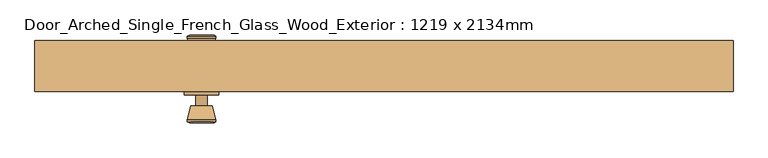
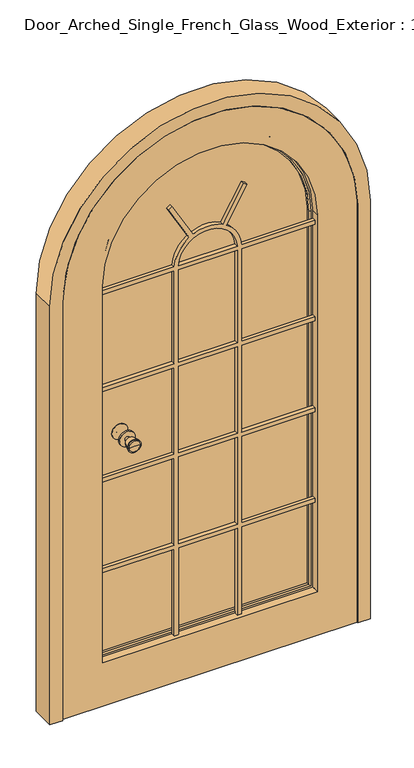
"""IFC4 building model written with IfcOpenShell, lengths in millimetres: door geometry, Door_Arched_Single_French_Glass_Wood_Exterior : 1219 x 2134mm."""

from ifc_helpers import new_model, si_unit, point, frame, frame_2d, origin, place, context, project, spatial, polyline, circle_curve, ellipse_curve, trimmed, segment, composite_curve, outline, extrude, source, transform, mapped, element, save
from ifc_brep_helpers import plane_surface, cylinder_surface, revolved_surface, advanced_brep


def door_arched_single_french_glass_wood_exterior_1219_x_2134mm_7a906126(model_context):
    return source(origin(), model_context, "Body", "SolidModel", [
        advanced_brep(
        [(-318.5, -5.7, 1050.0), (-308.5, -5.7, 1050.0), (-328.5, -5.7, 1050.0), (-298.0241324, -54.7, 1050.0), (-318.5, -54.7, 1050.0), (-338.9758676, -54.7, 1050.0), (-293.5, -52.8721319, 1050.0), (-343.5, -52.8721319, 1050.0), (-293.5, -49.4084537, 1050.0), (-343.5, -49.4084537, 1050.0), (-299.863764, -24.7, 1050.0), (-337.136236, -24.7, 1050.0), (-308.5, -24.7, 1050.0), (-328.5, -24.7, 1050.0)],
        [
            (0, 1),
            (1, 2, circle_curve(frame((-318.5, -5.7, 1050.0), z_axis=(0.0, 1.0, 0.0), x_axis=(-1.0, 0.0, 0.0)), 10.0)),
            (2, 0),
            (2, 1, circle_curve(frame((-318.5, -5.7, 1050.0), z_axis=(0.0, 1.0, 0.0), x_axis=(-1.0, 0.0, 0.0)), 10.0)),
            (3, 4),
            (4, 5),
            (5, 3, circle_curve(frame((-318.5, -54.7, 1050.0), z_axis=(0.0, -1.0, 0.0), x_axis=(-1.0, 0.0, 0.0)), 20.4758676)),
            (3, 5, circle_curve(frame((-318.5, -54.7, 1050.0), z_axis=(0.0, -1.0, 0.0), x_axis=(-1.0, 0.0, 0.0)), 20.4758676)),
            (6, 3),
            (5, 7),
            (7, 6, circle_curve(frame((-318.5, -52.8721319, 1050.0), z_axis=(0.0, -1.0, 0.0), x_axis=(-1.0, 0.0, 0.0)), 25.0)),
            (6, 7, circle_curve(frame((-318.5, -52.8721319, 1050.0), z_axis=(0.0, -1.0, 0.0), x_axis=(-1.0, 0.0, 0.0)), 25.0)),
            (8, 6),
            (7, 9),
            (9, 8, circle_curve(frame((-318.5, -49.4084537, 1050.0), z_axis=(0.0, -1.0, 0.0), x_axis=(-1.0, 0.0, 0.0)), 25.0)),
            (8, 9, circle_curve(frame((-318.5, -49.4084537, 1050.0), z_axis=(0.0, -1.0, 0.0), x_axis=(-1.0, 0.0, 0.0)), 25.0)),
            (10, 8),
            (9, 11),
            (11, 10, circle_curve(frame((-318.5, -24.7, 1050.0), z_axis=(0.0, -1.0, 0.0), x_axis=(-1.0, 0.0, 0.0)), 18.636236)),
            (10, 11, circle_curve(frame((-318.5, -24.7, 1050.0), z_axis=(0.0, -1.0, 0.0), x_axis=(-1.0, 0.0, 0.0)), 18.636236)),
            (12, 10),
            (11, 13),
            (13, 12, circle_curve(frame((-318.5, -24.7, 1050.0), z_axis=(0.0, -1.0, 0.0), x_axis=(-1.0, 0.0, 0.0)), 10.0)),
            (12, 13, circle_curve(frame((-318.5, -24.7, 1050.0), z_axis=(0.0, -1.0, 0.0), x_axis=(-1.0, 0.0, 0.0)), 10.0)),
            (1, 12),
            (13, 2),
        ],
        [
            plane_surface(frame((-318.5, -5.7, 1050.0), z_axis=(0.0, 1.0, 0.0), x_axis=(-1.0, 0.0, 0.0))),
            plane_surface(frame((-318.5, -54.7, 1050.0), z_axis=(0.0, -1.0, 0.0), x_axis=(-1.0, 0.0, 0.0))),
            revolved_surface(polyline([(-338.9758676, -54.7, 1050.0), (-343.5, -52.8721319, 1050.0)]), (-318.5, -5.7, 1050.0), (0.0, 1.0, 0.0)),
            cylinder_surface(frame((-318.5, -5.7, 1050.0), z_axis=(0.0, 1.0, 0.0), x_axis=(-1.0, 0.0, 0.0)), 25.0),
            revolved_surface(polyline([(-343.5, -49.4084537, 1050.0), (-337.136236, -24.7, 1050.0)]), (-318.5, -5.7, 1050.0), (0.0, 1.0, 0.0)),
            plane_surface(frame((-318.5, -24.7, 1050.0), z_axis=(0.0, 1.0, 0.0), x_axis=(-1.0, 0.0, 0.0))),
            cylinder_surface(frame((-318.5, -5.7, 1050.0), z_axis=(0.0, 1.0, 0.0), x_axis=(-1.0, 0.0, 0.0)), 10.0),
        ],
        [
            (0, [[1, 2, 3]]),
            (0, [[-3, 4, -1]]),
            (1, [[5, 6, 7]]),
            (1, [[-6, -5, 8]]),
            (2, [[9, -7, 10, 11]]),
            (2, [[-10, -8, -9, 12]]),
            (3, [[13, -11, 14, 15]]),
            (3, [[-14, -12, -13, 16]]),
            (4, [[17, -15, 18, 19]]),
            (4, [[-18, -16, -17, 20]]),
            (5, [[21, -19, 22, 23]]),
            (5, [[-22, -20, -21, 24]]),
            (6, [[25, -23, 26, -2]]),
            (6, [[-26, -24, -25, -4]]),
        ],
    ),
        extrude(outline(composite_curve([segment(trimmed(circle_curve(frame_2d((1050.0, -318.5)), 30.0), [point((1050.0, -348.5))], [point((1050.0, -288.5))], False, "CARTESIAN"), True, "CONTINUOUS"), segment(trimmed(circle_curve(frame_2d((1050.0, -318.5)), 30.0), [point((1050.0, -288.5))], [point((1050.0, -348.5))], False, "CARTESIAN"), True, "CONTINUOUS")], self_intersect=False)), frame((0.0, -5.7, 0.0), z_axis=(0.0, 1.0, 0.0), x_axis=(0.0, 0.0, 1.0)), (0.0, 0.0, 1.0), 6.0),
        advanced_brep(
        [(-318.5, 50.3, 1050.0), (-328.5, 50.3, 1050.0), (-308.5, 50.3, 1050.0), (-298.0241324, 99.3, 1050.0), (-338.9758676, 99.3, 1050.0), (-318.5, 99.3, 1050.0), (-293.5, 97.4721319, 1050.0), (-343.5, 97.4721319, 1050.0), (-293.5, 94.0084537, 1050.0), (-343.5, 94.0084537, 1050.0), (-299.863764, 69.3, 1050.0), (-337.136236, 69.3, 1050.0), (-308.5, 69.3, 1050.0), (-328.5, 69.3, 1050.0)],
        [
            (0, 1),
            (1, 2, circle_curve(frame((-318.5, 50.3, 1050.0), z_axis=(0.0, -1.0, 0.0), x_axis=(-1.0, 0.0, 0.0)), 10.0)),
            (2, 0),
            (2, 1, circle_curve(frame((-318.5, 50.3, 1050.0), z_axis=(0.0, -1.0, 0.0), x_axis=(-1.0, 0.0, 0.0)), 10.0)),
            (3, 4, circle_curve(frame((-318.5, 99.3, 1050.0), z_axis=(0.0, 1.0, 0.0), x_axis=(-1.0, 0.0, 0.0)), 20.4758676)),
            (4, 5),
            (5, 3),
            (4, 3, circle_curve(frame((-318.5, 99.3, 1050.0), z_axis=(0.0, 1.0, 0.0), x_axis=(-1.0, 0.0, 0.0)), 20.4758676)),
            (6, 7, circle_curve(frame((-318.5, 97.4721319, 1050.0), z_axis=(0.0, 1.0, 0.0), x_axis=(-1.0, 0.0, 0.0)), 25.0)),
            (7, 4),
            (3, 6),
            (7, 6, circle_curve(frame((-318.5, 97.4721319, 1050.0), z_axis=(0.0, 1.0, 0.0), x_axis=(-1.0, 0.0, 0.0)), 25.0)),
            (8, 9, circle_curve(frame((-318.5, 94.0084537, 1050.0), z_axis=(0.0, 1.0, 0.0), x_axis=(-1.0, 0.0, 0.0)), 25.0)),
            (9, 7),
            (6, 8),
            (9, 8, circle_curve(frame((-318.5, 94.0084537, 1050.0), z_axis=(0.0, 1.0, 0.0), x_axis=(-1.0, 0.0, 0.0)), 25.0)),
            (10, 11, circle_curve(frame((-318.5, 69.3, 1050.0), z_axis=(0.0, 1.0, 0.0), x_axis=(-1.0, 0.0, 0.0)), 18.636236)),
            (11, 9),
            (8, 10),
            (11, 10, circle_curve(frame((-318.5, 69.3, 1050.0), z_axis=(0.0, 1.0, 0.0), x_axis=(-1.0, 0.0, 0.0)), 18.636236)),
            (12, 13, circle_curve(frame((-318.5, 69.3, 1050.0), z_axis=(0.0, 1.0, 0.0), x_axis=(-1.0, 0.0, 0.0)), 10.0)),
            (13, 11),
            (10, 12),
            (13, 12, circle_curve(frame((-318.5, 69.3, 1050.0), z_axis=(0.0, 1.0, 0.0), x_axis=(-1.0, 0.0, 0.0)), 10.0)),
            (1, 13),
            (12, 2),
        ],
        [
            plane_surface(frame((-318.5, 50.3, 1050.0), z_axis=(0.0, -1.0, 0.0), x_axis=(-1.0, 0.0, 0.0))),
            plane_surface(frame((-318.5, 99.3, 1050.0), z_axis=(0.0, 1.0, 0.0), x_axis=(-1.0, 0.0, 0.0))),
            revolved_surface(polyline([(-338.9758676, 99.3, 1050.0), (-343.5, 97.4721319, 1050.0)]), (-318.5, 50.3, 1050.0), (0.0, -1.0, 0.0)),
            cylinder_surface(frame((-318.5, 50.3, 1050.0), z_axis=(0.0, -1.0, 0.0), x_axis=(-1.0, 0.0, 0.0)), 25.0),
            revolved_surface(polyline([(-343.5, 94.0084537, 1050.0), (-337.136236, 69.3, 1050.0)]), (-318.5, 50.3, 1050.0), (0.0, -1.0, 0.0)),
            plane_surface(frame((-318.5, 69.3, 1050.0), z_axis=(0.0, -1.0, 0.0), x_axis=(-1.0, 0.0, 0.0))),
            cylinder_surface(frame((-318.5, 50.3, 1050.0), z_axis=(0.0, -1.0, 0.0), x_axis=(-1.0, 0.0, 0.0)), 10.0),
        ],
        [
            (0, [[1, 2, 3]]),
            (0, [[-3, 4, -1]]),
            (1, [[5, 6, 7]]),
            (1, [[8, -7, -6]]),
            (2, [[9, 10, -5, 11]]),
            (2, [[12, -11, -8, -10]]),
            (3, [[13, 14, -9, 15]]),
            (3, [[16, -15, -12, -14]]),
            (4, [[17, 18, -13, 19]]),
            (4, [[20, -19, -16, -18]]),
            (5, [[21, 22, -17, 23]]),
            (5, [[24, -23, -20, -22]]),
            (6, [[-2, 25, -21, 26]]),
            (6, [[-4, -26, -24, -25]]),
        ],
    ),
        extrude(outline(composite_curve([segment(trimmed(circle_curve(frame_2d((1050.0, -318.5)), 30.0), [point((1050.0, -348.5))], [point((1050.0, -288.5))], False, "CARTESIAN"), True, "CONTINUOUS"), segment(trimmed(circle_curve(frame_2d((1050.0, -318.5)), 30.0), [point((1050.0, -288.5))], [point((1050.0, -348.5))], False, "CARTESIAN"), True, "CONTINUOUS")], self_intersect=False)), frame((0.0, 44.3, 0.0), z_axis=(0.0, 1.0, 0.0), x_axis=(0.0, 0.0, 1.0)), (0.0, 0.0, 1.0), 6.0),
        advanced_brep(
        [(539.1, 89.3, 0.0), (609.6, 89.3, 0.0), (609.6, 0.3, 0.0), (561.1, 0.3, 0.0), (561.1, 47.3, 0.0), (539.1, 47.3, 0.0), (539.1, 89.3, 1678.6), (-539.1, 89.3, 1678.6), (-539.1, 89.3, 0.0), (-609.6, 89.3, 0.0), (-609.6, 89.3, 1678.6), (609.6, 89.3, 1678.6), (609.6, 0.3, 1678.6), (-609.6, 0.3, 1678.6), (-609.6, 0.3, 0.0), (-561.1, 0.3, 0.0), (-561.1, 0.3, 1678.6), (561.1, 0.3, 1678.6), (561.1, 47.3, 1678.6), (-561.1, 47.3, 1678.6), (-561.1, 47.3, 0.0), (-539.1, 47.3, 0.0), (-539.1, 47.3, 1678.6), (539.1, 47.3, 1678.6)],
        [
            (0, 1),
            (1, 2),
            (2, 3),
            (3, 4),
            (4, 5),
            (5, 0),
            (0, 6),
            (6, 7, circle_curve(frame((0.0, 89.3, 1678.6), z_axis=(0.0, -1.0, 0.0), x_axis=(1.0, 0.0, 0.0)), 539.1)),
            (7, 8),
            (8, 9),
            (9, 10),
            (10, 11, circle_curve(frame((0.0, 89.3, 1678.6), z_axis=(0.0, 1.0, 0.0), x_axis=(1.0, 0.0, 0.0)), 609.6)),
            (11, 1),
            (11, 12),
            (12, 2),
            (12, 13, circle_curve(frame((0.0, 0.3, 1678.6), z_axis=(0.0, -1.0, 0.0), x_axis=(1.0, 0.0, 0.0)), 609.6)),
            (13, 14),
            (14, 15),
            (15, 16),
            (16, 17, circle_curve(frame((0.0, 0.3, 1678.6), z_axis=(0.0, 1.0, 0.0), x_axis=(1.0, 0.0, 0.0)), 561.1)),
            (17, 3),
            (17, 18),
            (18, 4),
            (18, 19, circle_curve(frame((0.0, 47.3, 1678.6), z_axis=(0.0, -1.0, 0.0), x_axis=(1.0, 0.0, 0.0)), 561.1)),
            (19, 20),
            (20, 21),
            (21, 22),
            (22, 23, circle_curve(frame((0.0, 47.3, 1678.6), z_axis=(0.0, 1.0, 0.0), x_axis=(1.0, 0.0, 0.0)), 539.1)),
            (23, 5),
            (23, 6),
            (7, 22),
            (21, 8),
            (20, 15),
            (14, 9),
            (13, 10),
            (19, 16),
        ],
        [
            plane_surface(frame((603.1, -9.1123976, 0.0), z_axis=(0.0, 0.0, -1.0), x_axis=(1.0, 0.0, 0.0))),
            plane_surface(frame((539.1, 89.3, 0.0), z_axis=(0.0, 1.0, 0.0), x_axis=(0.0, 0.0, 1.0))),
            plane_surface(frame((609.6, 89.3, 0.0), z_axis=(1.0, 0.0, 0.0), x_axis=(0.0, 0.0, 1.0))),
            plane_surface(frame((609.6, 0.3, 0.0), z_axis=(0.0, -1.0, 0.0), x_axis=(0.0, 0.0, 1.0))),
            plane_surface(frame((561.1, 0.3, 0.0), z_axis=(-1.0, 0.0, 0.0), x_axis=(0.0, 0.0, 1.0))),
            plane_surface(frame((561.1, 47.3, 0.0), z_axis=(0.0, -1.0, 0.0), x_axis=(0.0, 0.0, 1.0))),
            plane_surface(frame((539.1, 47.3, 0.0), z_axis=(-1.0, 0.0, 0.0), x_axis=(0.0, 0.0, 1.0))),
            plane_surface(frame((-539.1, 47.3, 1678.6), z_axis=(1.0, 0.0, 0.0), x_axis=(0.0, 0.0, -1.0))),
            plane_surface(frame((-603.1, -9.1123976, 0.0), z_axis=(0.0, 0.0, -1.0), x_axis=(-1.0, 0.0, 0.0))),
            plane_surface(frame((-609.6, 89.3, 1678.6), z_axis=(-1.0, 0.0, 0.0), x_axis=(0.0, 0.0, -1.0))),
            plane_surface(frame((-561.1, 0.3, 1678.6), z_axis=(1.0, 0.0, 0.0), x_axis=(0.0, 0.0, -1.0))),
            cylinder_surface(frame((0.0, 89.3, 1678.6), z_axis=(0.0, -1.0, 0.0), x_axis=(1.0, 0.0, 0.0)), 609.6),
            revolved_surface(polyline([(561.1, 0.29999999999999716, 1678.6), (561.1, 47.3, 1678.6)]), (0.0, 89.3, 1678.6), (0.0, -1.0, 0.0)),
            revolved_surface(polyline([(539.1, 47.3, 1678.6), (539.1, 89.3, 1678.6)]), (0.0, 89.3, 1678.6), (0.0, -1.0, 0.0)),
        ],
        [
            (0, [[1, 2, 3, 4, 5, 6]]),
            (1, [[-1, 7, 8, 9, 10, 11, 12, 13]]),
            (2, [[-2, -13, 14, 15]]),
            (3, [[-3, -15, 16, 17, 18, 19, 20, 21]]),
            (4, [[-4, -21, 22, 23]]),
            (5, [[-5, -23, 24, 25, 26, 27, 28, 29]]),
            (6, [[-6, -29, 30, -7]]),
            (7, [[31, -27, 32, -9]]),
            (8, [[-32, -26, 33, -18, 34, -10]]),
            (9, [[35, -11, -34, -17]]),
            (10, [[36, -19, -33, -25]]),
            (11, [[-16, -14, -12, -35]]),
            (12, [[-24, -22, -20, -36]]),
            (13, [[-8, -30, -28, -31]]),
        ],
    ),
        extrude(outline(composite_curve([segment(trimmed(circle_curve(frame_2d((1692.1, 0.0)), 253.5), [point((1896.740356, 149.6147543))], [point((1905.7961472, 136.3679092))], False, "CARTESIAN"), True, "CONTINUOUS"), segment(polyline([(1905.7961472, 136.3679092), (1768.2345335, 56.9466745)]), True, "CONTINUOUS"), segment(trimmed(circle_curve(frame_2d((1653.6, 0.0)), 128.0), [point((1768.2345335, 56.9466745))], [point((1768.2345335, -56.9466745))], False, "CARTESIAN"), True, "CONTINUOUS"), segment(polyline([(1768.2345335, -56.9466745), (1905.7961472, -136.3679092)]), True, "CONTINUOUS"), segment(trimmed(circle_curve(frame_2d((1692.1, 0.0)), 253.5), [point((1905.7961472, -136.3679092))], [point((1896.740356, -149.6147543))], False, "CARTESIAN"), True, "CONTINUOUS"), segment(polyline([(1896.740356, -149.6147543), (1760.2345335, -70.8030809)]), True, "CONTINUOUS"), segment(trimmed(circle_curve(frame_2d((1653.6, 0.0)), 128.0), [point((1760.2345335, -70.8030809))], [point((1661.6, -127.7497554))], False, "CARTESIAN"), True, "CONTINUOUS"), segment(polyline([(1661.6, -127.7497554), (1661.6, -408.1), (1645.6, -408.1), (1645.6, -128.0), (1273.5, -128.0), (1273.5, -408.1), (1257.5, -408.1), (1257.5, -128.0), (909.0, -128.0), (909.0, -408.1), (893.0, -408.1), (893.0, -128.0), (544.5, -128.0), (544.5, -408.1), (528.5, -408.1), (528.5, -128.0), (179.0, -128.0), (179.0, -112.0), (528.5, -112.0), (528.5, 112.0), (179.0, 112.0), (179.0, 128.0), (528.5, 128.0), (528.5, 408.1), (544.5, 408.1), (544.5, 128.0), (893.0, 128.0), (893.0, 408.1), (909.0, 408.1), (909.0, 128.0), (1257.5, 128.0), (1257.5, 408.1), (1273.5, 408.1), (1273.5, 128.0), (1645.6, 128.0), (1645.6, 408.1), (1661.6, 408.1), (1661.6, 127.7497554)]), True, "CONTINUOUS"), segment(trimmed(circle_curve(frame_2d((1653.6, 0.0)), 128.0), [point((1661.6, 127.7497554))], [point((1760.2345335, 70.8030809))], False, "CARTESIAN"), True, "CONTINUOUS"), segment(polyline([(1760.2345335, 70.8030809), (1896.740356, 149.6147543)]), True, "CONTINUOUS")], self_intersect=False), holes=[polyline([(893.0, -112.0), (893.0, 112.0), (544.5, 112.0), (544.5, -112.0), (893.0, -112.0)]), polyline([(1257.5, 112.0), (909.0, 112.0), (909.0, -112.0), (1257.5, -112.0), (1257.5, 112.0)]), composite_curve([segment(trimmed(circle_curve(frame_2d((1653.6, 0.0)), 112.0), [point((1661.6, -111.7139204))], [point((1661.6, 111.7139204))], True, "CARTESIAN"), True, "CONTINUOUS"), segment(polyline([(1661.6, 111.7139204), (1661.6, -111.7139204)]), True, "CONTINUOUS")], self_intersect=False), polyline([(1645.6, -112.0), (1645.6, 112.0), (1273.5, 112.0), (1273.5, -112.0), (1645.6, -112.0)])]), frame((0.0, 15.1515468, 0.0), z_axis=(0.0, 1.0, 0.0), x_axis=(0.0, 0.0, 1.0)), (0.0, 0.0, 1.0), 14.5359085),
        extrude(outline(composite_curve([segment(polyline([(4.0, 558.1), (1727.8950302, 558.1)]), True, "CONTINUOUS"), segment(trimmed(circle_curve(frame_2d((1678.6, 0.0)), 560.2727996), [point((1727.8950302, 558.1))], [point((1715.9714663, -559.0250294))], False, "CARTESIAN"), True, "CONTINUOUS"), segment(polyline([(1715.9714663, -559.0250294), (4.0, -559.0250294), (4.0, 558.1)]), True, "CONTINUOUS")], self_intersect=False), holes=[composite_curve([segment(polyline([(179.0, -408.1), (1692.1, -408.1)]), True, "CONTINUOUS"), segment(trimmed(circle_curve(frame_2d((1692.1, 0.0)), 408.1), [point((1692.1, -408.1))], [point((1692.1, 408.1))], True, "CARTESIAN"), True, "CONTINUOUS"), segment(polyline([(1692.1, 408.1), (179.0, 408.1), (179.0, -408.1)]), True, "CONTINUOUS")], self_intersect=False)]), frame((0.0, 0.3, 0.0), z_axis=(0.0, 1.0, 0.0), x_axis=(0.0, 0.0, 1.0)), (0.0, 0.0, 1.0), 44.0),
        extrude(outline(composite_curve([segment(polyline([(179.0, -408.1), (179.0, 408.1), (1692.1, 408.1)]), True, "CONTINUOUS"), segment(trimmed(circle_curve(frame_2d((1692.1, 0.0)), 408.1), [point((1692.1, 408.1))], [point((1692.1, -408.1))], False, "CARTESIAN"), True, "CONTINUOUS"), segment(polyline([(1692.1, -408.1), (179.0, -408.1)]), True, "CONTINUOUS")], self_intersect=False)), frame((0.0, 46.0, 0.0), z_axis=(0.0, 1.0, 0.0), x_axis=(0.0, 0.0, 1.0)), (0.0, 0.0, 1.0), 24.0),
        advanced_brep(
        [(-416.1, 84.0, 171.0), (-416.1, 80.0, 171.0), (-416.1, 80.0, 1692.1), (-416.1, 84.0, 1692.1), (-414.1, 86.0, 173.0), (-414.1, 86.0, 1692.1), (-396.1, 81.0, 191.0), (-401.1, 86.0, 186.0), (-401.1, 86.0, 1692.1), (-396.1, 81.0, 1692.1), (-396.1, 70.0, 191.0), (-396.1, 70.0, 1692.1), (-408.1, 80.0, 179.0), (-408.1, 70.0, 179.0), (-408.1, 70.0, 1692.1), (-408.1, 80.0, 1692.1), (416.1, 84.0, 1692.1), (416.1, 80.0, 1692.1), (414.1, 86.0, 1692.1), (414.1, 86.0, 173.0), (401.1, 86.0, 1692.1), (401.1, 86.0, 186.0), (396.1, 81.0, 1692.1), (396.1, 70.0, 1692.1), (408.1, 70.0, 1692.1), (408.1, 70.0, 179.0), (396.1, 70.0, 191.0), (408.1, 80.0, 1692.1), (416.1, 80.0, 171.0), (408.1, 80.0, 179.0), (416.1, 84.0, 171.0), (396.1, 81.0, 191.0)],
        [
            (0, 1),
            (1, 2),
            (2, 3),
            (3, 0),
            (4, 0, ellipse_curve(frame((-414.1, 84.0, 173.0), z_axis=(-0.7071067811865475, 0.0, 0.7071067811865475), x_axis=(-0.7071067811865474, 0.0, -0.7071067811865476)), 2.8284271, 2.0)),
            (3, 5, circle_curve(frame((-414.1, 84.0, 1692.1), z_axis=(0.0, 0.0, -1.0), x_axis=(-1.0, 0.0, 0.0)), 2.0)),
            (5, 4),
            (6, 7, ellipse_curve(frame((-401.1, 81.0, 186.0), z_axis=(-0.7071067811865475, 0.0, 0.7071067811865475), x_axis=(-0.7071067811865474, 0.0, -0.7071067811865476)), 7.0710678, 5.0)),
            (7, 8),
            (8, 9, circle_curve(frame((-401.1, 81.0, 1692.1), z_axis=(0.0, 0.0, -1.0), x_axis=(-1.0, 0.0, 0.0)), 5.0)),
            (9, 6),
            (10, 6),
            (9, 11),
            (11, 10),
            (12, 13),
            (13, 14),
            (14, 15),
            (15, 12),
            (16, 3, circle_curve(frame((0.0, 84.0, 1692.1), z_axis=(0.0, -1.0, 0.0), x_axis=(-1.0, 0.0, 0.0)), 416.1)),
            (2, 17, circle_curve(frame((0.0, 80.0, 1692.1), z_axis=(0.0, 1.0, 0.0), x_axis=(-1.0, 0.0, 0.0)), 416.1)),
            (17, 16),
            (18, 5, circle_curve(frame((0.0, 86.0, 1692.1), z_axis=(0.0, -1.0, 0.0), x_axis=(-1.0, 0.0, 0.0)), 414.1)),
            (16, 18, circle_curve(frame((414.1, 84.0, 1692.1), z_axis=(0.0, 0.0, 1.0), x_axis=(1.0, 0.0, 0.0)), 2.0)),
            (18, 19),
            (19, 4),
            (20, 8, circle_curve(frame((0.0, 86.0, 1692.1), z_axis=(0.0, -1.0, 0.0), x_axis=(-1.0, 0.0, 0.0)), 401.1)),
            (7, 21),
            (21, 20),
            (22, 9, circle_curve(frame((0.0, 81.0, 1692.1), z_axis=(0.0, -1.0, 0.0), x_axis=(-1.0, 0.0, 0.0)), 396.1)),
            (20, 22, circle_curve(frame((401.1, 81.0, 1692.1), z_axis=(0.0, 0.0, 1.0), x_axis=(1.0, 0.0, 0.0)), 5.0)),
            (23, 11, circle_curve(frame((0.0, 70.0, 1692.1), z_axis=(0.0, -1.0, 0.0), x_axis=(-1.0, 0.0, 0.0)), 396.1)),
            (22, 23),
            (24, 14, circle_curve(frame((0.0, 70.0, 1692.1), z_axis=(0.0, -1.0, 0.0), x_axis=(-1.0, 0.0, 0.0)), 408.1)),
            (13, 25),
            (25, 24),
            (23, 26),
            (26, 10),
            (27, 15, circle_curve(frame((0.0, 80.0, 1692.1), z_axis=(0.0, -1.0, 0.0), x_axis=(-1.0, 0.0, 0.0)), 408.1)),
            (24, 27),
            (1, 28),
            (28, 17),
            (27, 29),
            (29, 12),
            (28, 30),
            (30, 16),
            (30, 19, ellipse_curve(frame((414.1, 84.0, 173.0), z_axis=(0.7071067811865475, 0.0, 0.7071067811865475), x_axis=(-0.7071067811865474, 0.0, 0.7071067811865476)), 2.8284271, 2.0)),
            (21, 31, ellipse_curve(frame((401.1, 81.0, 186.0), z_axis=(0.7071067811865475, 0.0, 0.7071067811865475), x_axis=(-0.7071067811865474, 0.0, 0.7071067811865476)), 7.0710678, 5.0)),
            (31, 22),
            (31, 26),
            (25, 29),
            (0, 30),
            (6, 31),
        ],
        [
            plane_surface(frame((-416.1, 80.0, 171.0), z_axis=(-1.0, 0.0, 0.0), x_axis=(0.0, 0.0, 1.0))),
            cylinder_surface(frame((-414.1, 84.0, 179.0), z_axis=(0.0, 0.0, -1.0), x_axis=(-1.0, 0.0, 0.0)), 2.0),
            cylinder_surface(frame((-401.1, 81.0, 179.0), z_axis=(0.0, 0.0, -1.0), x_axis=(-1.0, 0.0, 0.0)), 5.0),
            plane_surface(frame((-396.1, 81.0, 191.0), z_axis=(1.0, 0.0, 0.0), x_axis=(0.0, 0.0, 1.0))),
            plane_surface(frame((-408.1, 70.0, 179.0), z_axis=(-1.0, 0.0, 0.0), x_axis=(0.0, 0.0, 1.0))),
            cylinder_surface(frame((0.0, 80.0, 1692.1), z_axis=(0.0, 1.0, 0.0), x_axis=(-1.0, 0.0, 0.0)), 416.1),
            revolved_surface(trimmed(ellipse_curve(frame((-414.1, 84.0, 1692.1), z_axis=(0.0, 0.0, -1.0), x_axis=(-1.0, 0.0, 0.0)), 2.0, 2.0), [point((-416.1, 84.0, 1692.1))], [point((-414.1, 86.0, 1692.1))], True, "CARTESIAN"), (0.0, 80.0, 1692.1), (0.0, 1.0, 0.0)),
            plane_surface(frame((0.0, 86.0, 1692.1), z_axis=(0.0, 1.0, 0.0), x_axis=(-1.0, 0.0, 0.0))),
            revolved_surface(trimmed(ellipse_curve(frame((-401.1, 81.0, 1692.1), z_axis=(0.0, 0.0, -1.0), x_axis=(-1.0, 0.0, 0.0)), 5.0, 5.0), [point((-401.1, 86.0, 1692.1))], [point((-396.1, 81.0, 1692.1))], True, "CARTESIAN"), (0.0, 80.0, 1692.1), (0.0, 1.0, 0.0)),
            revolved_surface(polyline([(-396.1, 81.0, 1692.1), (-396.1, 70.0, 1692.1)]), (0.0, 80.0, 1692.1), (0.0, 1.0, 0.0)),
            plane_surface(frame((0.0, 70.0, 1692.1), z_axis=(0.0, -1.0, 0.0), x_axis=(-1.0, 0.0, 0.0))),
            cylinder_surface(frame((0.0, 80.0, 1692.1), z_axis=(0.0, 1.0, 0.0), x_axis=(-1.0, 0.0, 0.0)), 408.1),
            plane_surface(frame((0.0, 80.0, 1692.1), z_axis=(0.0, -1.0, 0.0), x_axis=(-1.0, 0.0, 0.0))),
            plane_surface(frame((416.1, 80.0, 1692.1), z_axis=(1.0, 0.0, 0.0), x_axis=(0.0, 0.0, -1.0))),
            cylinder_surface(frame((414.1, 84.0, 1692.1), z_axis=(0.0, 0.0, 1.0), x_axis=(1.0, 0.0, 0.0)), 2.0),
            cylinder_surface(frame((401.1, 81.0, 1692.1), z_axis=(0.0, 0.0, 1.0), x_axis=(1.0, 0.0, 0.0)), 5.0),
            plane_surface(frame((396.1, 81.0, 1692.1), z_axis=(-1.0, 0.0, 0.0), x_axis=(0.0, 0.0, -1.0))),
            plane_surface(frame((408.1, 70.0, 1692.1), z_axis=(1.0, 0.0, 0.0), x_axis=(0.0, 0.0, -1.0))),
            plane_surface(frame((416.1, 80.0, 171.0), z_axis=(0.0, 0.0, -1.0), x_axis=(-1.0, 0.0, 0.0))),
            cylinder_surface(frame((408.1, 84.0, 173.0), z_axis=(1.0, 0.0, 0.0), x_axis=(0.0, 0.0, -1.0)), 2.0),
            cylinder_surface(frame((408.1, 81.0, 186.0), z_axis=(1.0, 0.0, 0.0), x_axis=(0.0, 0.0, -1.0)), 5.0),
            plane_surface(frame((396.1, 81.0, 191.0), z_axis=(0.0, 0.0, 1.0), x_axis=(-1.0, 0.0, 0.0))),
            plane_surface(frame((408.1, 70.0, 179.0), z_axis=(0.0, 0.0, -1.0), x_axis=(-1.0, 0.0, 0.0))),
        ],
        [
            (0, [[1, 2, 3, 4]]),
            (1, [[5, -4, 6, 7]]),
            (2, [[8, 9, 10, 11]]),
            (3, [[12, -11, 13, 14]]),
            (4, [[15, 16, 17, 18]]),
            (5, [[19, -3, 20, 21]]),
            (6, [[22, -6, -19, 23]]),
            (7, [[24, 25, -7, -22], [26, -9, 27, 28]]),
            (8, [[29, -10, -26, 30]]),
            (9, [[31, -13, -29, 32]]),
            (10, [[33, -16, 34, 35], [36, 37, -14, -31]]),
            (11, [[38, -17, -33, 39]]),
            (12, [[-20, -2, 40, 41], [42, 43, -18, -38]]),
            (13, [[-21, -41, 44, 45]]),
            (14, [[-23, -45, 46, -24]]),
            (15, [[-30, -28, 47, 48]]),
            (16, [[-32, -48, 49, -36]]),
            (17, [[-39, -35, 50, -42]]),
            (18, [[-44, -40, -1, 51]]),
            (19, [[-46, -51, -5, -25]]),
            (20, [[-47, -27, -8, 52]]),
            (21, [[-49, -52, -12, -37]]),
            (22, [[-50, -34, -15, -43]]),
        ],
    ),
        advanced_brep(
        [(416.1, 32.0, 171.0), (416.1, 36.0, 171.0), (416.1, 36.0, 1692.1), (416.1, 32.0, 1692.1), (414.1, 30.0, 173.0), (414.1, 30.0, 1692.1), (396.1, 35.0, 191.0), (401.1, 30.0, 186.0), (401.1, 30.0, 1692.1), (396.1, 35.0, 1692.1), (396.1, 46.0, 191.0), (396.1, 46.0, 1692.1), (408.1, 36.0, 179.0), (408.1, 46.0, 179.0), (408.1, 46.0, 1692.1), (408.1, 36.0, 1692.1), (-416.1, 32.0, 1692.1), (-416.1, 36.0, 1692.1), (-414.1, 30.0, 1692.1), (-414.1, 30.0, 173.0), (-401.1, 30.0, 1692.1), (-401.1, 30.0, 186.0), (-396.1, 35.0, 1692.1), (-396.1, 46.0, 1692.1), (-408.1, 46.0, 1692.1), (-408.1, 46.0, 179.0), (-396.1, 46.0, 191.0), (-408.1, 36.0, 1692.1), (-416.1, 36.0, 171.0), (-408.1, 36.0, 179.0), (-416.1, 32.0, 171.0), (-396.1, 35.0, 191.0)],
        [
            (0, 1),
            (1, 2),
            (2, 3),
            (3, 0),
            (4, 0, ellipse_curve(frame((414.1, 32.0, 173.0), z_axis=(0.7071067811865475, 0.0, 0.7071067811865475), x_axis=(0.7071067811865474, 0.0, -0.7071067811865476)), 2.8284271, 2.0)),
            (3, 5, circle_curve(frame((414.1, 32.0, 1692.1), z_axis=(0.0, 0.0, -1.0), x_axis=(1.0, 0.0, 0.0)), 2.0)),
            (5, 4),
            (6, 7, ellipse_curve(frame((401.1, 35.0, 186.0), z_axis=(0.7071067811865475, 0.0, 0.7071067811865475), x_axis=(0.7071067811865474, 0.0, -0.7071067811865476)), 7.0710678, 5.0)),
            (7, 8),
            (8, 9, circle_curve(frame((401.1, 35.0, 1692.1), z_axis=(0.0, 0.0, -1.0), x_axis=(1.0, 0.0, 0.0)), 5.0)),
            (9, 6),
            (10, 6),
            (9, 11),
            (11, 10),
            (12, 13),
            (13, 14),
            (14, 15),
            (15, 12),
            (16, 3, circle_curve(frame((0.0, 32.0, 1692.1), z_axis=(0.0, 1.0, 0.0), x_axis=(1.0, 0.0, 0.0)), 416.1)),
            (2, 17, circle_curve(frame((0.0, 36.0, 1692.1), z_axis=(0.0, -1.0, 0.0), x_axis=(1.0, 0.0, 0.0)), 416.1)),
            (17, 16),
            (18, 5, circle_curve(frame((0.0, 30.0, 1692.1), z_axis=(0.0, 1.0, 0.0), x_axis=(1.0, 0.0, 0.0)), 414.1)),
            (16, 18, circle_curve(frame((-414.1, 32.0, 1692.1), z_axis=(0.0, 0.0, 1.0), x_axis=(-1.0, 0.0, 0.0)), 2.0)),
            (18, 19),
            (19, 4),
            (20, 8, circle_curve(frame((0.0, 30.0, 1692.1), z_axis=(0.0, 1.0, 0.0), x_axis=(1.0, 0.0, 0.0)), 401.1)),
            (7, 21),
            (21, 20),
            (22, 9, circle_curve(frame((0.0, 35.0, 1692.1), z_axis=(0.0, 1.0, 0.0), x_axis=(1.0, 0.0, 0.0)), 396.1)),
            (20, 22, circle_curve(frame((-401.1, 35.0, 1692.1), z_axis=(0.0, 0.0, 1.0), x_axis=(-1.0, 0.0, 0.0)), 5.0)),
            (23, 11, circle_curve(frame((0.0, 46.0, 1692.1), z_axis=(0.0, 1.0, 0.0), x_axis=(1.0, 0.0, 0.0)), 396.1)),
            (22, 23),
            (24, 14, circle_curve(frame((0.0, 46.0, 1692.1), z_axis=(0.0, 1.0, 0.0), x_axis=(1.0, 0.0, 0.0)), 408.1)),
            (13, 25),
            (25, 24),
            (23, 26),
            (26, 10),
            (27, 15, circle_curve(frame((0.0, 36.0, 1692.1), z_axis=(0.0, 1.0, 0.0), x_axis=(1.0, 0.0, 0.0)), 408.1)),
            (24, 27),
            (1, 28),
            (28, 17),
            (27, 29),
            (29, 12),
            (28, 30),
            (30, 16),
            (30, 19, ellipse_curve(frame((-414.1, 32.0, 173.0), z_axis=(-0.7071067811865475, 0.0, 0.7071067811865475), x_axis=(0.7071067811865474, 0.0, 0.7071067811865476)), 2.8284271, 2.0)),
            (21, 31, ellipse_curve(frame((-401.1, 35.0, 186.0), z_axis=(-0.7071067811865475, 0.0, 0.7071067811865475), x_axis=(0.7071067811865474, 0.0, 0.7071067811865476)), 7.0710678, 5.0)),
            (31, 22),
            (31, 26),
            (25, 29),
            (0, 30),
            (6, 31),
        ],
        [
            plane_surface(frame((416.1, 36.0, 171.0), z_axis=(1.0, 0.0, 0.0), x_axis=(0.0, 0.0, 1.0))),
            cylinder_surface(frame((414.1, 32.0, 179.0), z_axis=(0.0, 0.0, -1.0), x_axis=(1.0, 0.0, 0.0)), 2.0),
            cylinder_surface(frame((401.1, 35.0, 179.0), z_axis=(0.0, 0.0, -1.0), x_axis=(1.0, 0.0, 0.0)), 5.0),
            plane_surface(frame((396.1, 35.0, 191.0), z_axis=(-1.0, 0.0, 0.0), x_axis=(0.0, 0.0, 1.0))),
            plane_surface(frame((408.1, 46.0, 179.0), z_axis=(1.0, 0.0, 0.0), x_axis=(0.0, 0.0, 1.0))),
            cylinder_surface(frame((0.0, 36.0, 1692.1), z_axis=(0.0, -1.0, 0.0), x_axis=(1.0, 0.0, 0.0)), 416.1),
            revolved_surface(trimmed(ellipse_curve(frame((414.1, 32.0, 1692.1), z_axis=(0.0, 0.0, -1.0), x_axis=(1.0, 0.0, 0.0)), 2.0, 2.0), [point((416.1, 32.0, 1692.1))], [point((414.1, 30.0, 1692.1))], True, "CARTESIAN"), (0.0, 36.0, 1692.1), (0.0, -1.0, 0.0)),
            plane_surface(frame((0.0, 30.0, 1692.1), z_axis=(0.0, -1.0, 0.0), x_axis=(1.0, 0.0, 0.0))),
            revolved_surface(trimmed(ellipse_curve(frame((401.1, 35.0, 1692.1), z_axis=(0.0, 0.0, -1.0), x_axis=(1.0, 0.0, 0.0)), 5.0, 5.0), [point((401.1, 30.0, 1692.1))], [point((396.1, 35.0, 1692.1))], True, "CARTESIAN"), (0.0, 36.0, 1692.1), (0.0, -1.0, 0.0)),
            revolved_surface(polyline([(396.1, 35.0, 1692.1), (396.1, 46.0, 1692.1)]), (0.0, 36.0, 1692.1), (0.0, -1.0, 0.0)),
            plane_surface(frame((0.0, 46.0, 1692.1), z_axis=(0.0, 1.0, 0.0), x_axis=(1.0, 0.0, 0.0))),
            cylinder_surface(frame((0.0, 36.0, 1692.1), z_axis=(0.0, -1.0, 0.0), x_axis=(1.0, 0.0, 0.0)), 408.1),
            plane_surface(frame((0.0, 36.0, 1692.1), z_axis=(0.0, 1.0, 0.0), x_axis=(1.0, 0.0, 0.0))),
            plane_surface(frame((-416.1, 36.0, 1692.1), z_axis=(-1.0, 0.0, 0.0), x_axis=(0.0, 0.0, -1.0))),
            cylinder_surface(frame((-414.1, 32.0, 1692.1), z_axis=(0.0, 0.0, 1.0), x_axis=(-1.0, 0.0, 0.0)), 2.0),
            cylinder_surface(frame((-401.1, 35.0, 1692.1), z_axis=(0.0, 0.0, 1.0), x_axis=(-1.0, 0.0, 0.0)), 5.0),
            plane_surface(frame((-396.1, 35.0, 1692.1), z_axis=(1.0, 0.0, 0.0), x_axis=(0.0, 0.0, -1.0))),
            plane_surface(frame((-408.1, 46.0, 1692.1), z_axis=(-1.0, 0.0, 0.0), x_axis=(0.0, 0.0, -1.0))),
            plane_surface(frame((-416.1, 36.0, 171.0), z_axis=(0.0, 0.0, -1.0), x_axis=(1.0, 0.0, 0.0))),
            cylinder_surface(frame((-408.1, 32.0, 173.0), z_axis=(-1.0, 0.0, 0.0), x_axis=(0.0, 0.0, -1.0)), 2.0),
            cylinder_surface(frame((-408.1, 35.0, 186.0), z_axis=(-1.0, 0.0, 0.0), x_axis=(0.0, 0.0, -1.0)), 5.0),
            plane_surface(frame((-396.1, 35.0, 191.0), z_axis=(0.0, 0.0, 1.0), x_axis=(1.0, 0.0, 0.0))),
            plane_surface(frame((-408.1, 46.0, 179.0), z_axis=(0.0, 0.0, -1.0), x_axis=(1.0, 0.0, 0.0))),
        ],
        [
            (0, [[1, 2, 3, 4]]),
            (1, [[5, -4, 6, 7]]),
            (2, [[8, 9, 10, 11]]),
            (3, [[12, -11, 13, 14]]),
            (4, [[15, 16, 17, 18]]),
            (5, [[19, -3, 20, 21]]),
            (6, [[22, -6, -19, 23]]),
            (7, [[24, 25, -7, -22], [26, -9, 27, 28]]),
            (8, [[29, -10, -26, 30]]),
            (9, [[31, -13, -29, 32]]),
            (10, [[33, -16, 34, 35], [36, 37, -14, -31]]),
            (11, [[38, -17, -33, 39]]),
            (12, [[-20, -2, 40, 41], [42, 43, -18, -38]]),
            (13, [[-21, -41, 44, 45]]),
            (14, [[-23, -45, 46, -24]]),
            (15, [[-30, -28, 47, 48]]),
            (16, [[-32, -48, 49, -36]]),
            (17, [[-39, -35, 50, -42]]),
            (18, [[-44, -40, -1, 51]]),
            (19, [[-46, -51, -5, -25]]),
            (20, [[-47, -27, -8, 52]]),
            (21, [[-49, -52, -12, -37]]),
            (22, [[-50, -34, -15, -43]]),
        ],
    ),
    ])


if __name__ == "__main__":
    model = new_model("IFC4")
    model_context = context("Model", 3, world=origin())
    ifc_project = project(units=[si_unit("LENGTHUNIT", "METRE", prefix="MILLI")], contexts=[model_context])
    site = spatial("IfcSite", under=ifc_project)
    building = spatial("IfcBuilding", under=site)
    placement = place(None, origin())
    door_arched_single_french_glass_wood_exterior_1219_x_2134mm_shape = door_arched_single_french_glass_wood_exterior_1219_x_2134mm_7a906126(model_context)
    element("IfcDoor", 1, ObjectType="Door_Arched_Single_French_Glass_Wood_Exterior : 1219 x 2134mm", at=placement, inside=building, context=model_context, shape_type="MappedRepresentation", body=[
        mapped(door_arched_single_french_glass_wood_exterior_1219_x_2134mm_shape, transform((0.0, 0.0, 0.0), x_axis=(1.0, 0.0, 0.0), y_axis=(0.0, 1.0, 0.0), z_axis=(0.0, 0.0, 1.0))),
    ])
    save(model, "model.ifc")

# Revit data of these elements
# Type "Door_Arched_Single_French_Glass_Wood_Exterior : 1219 x 2134mm"
#   Type Mark = "12"
#   Type Comments = "External Single"
#   Operation = "SingleSwingRight"
#   Keynote = "L20"
#   Analytic Construction = "<None>"
#   Wrap Layers (Int) from Ext = 0' - 6.98819"
#   Wrap Layers (Ext) from Ext = 0' - 4.03543"
#   Thickness = 0' - 1.73228"
#   Stile Shutting = 0' - 5.90551"
#   Stile - Top Rail = 0' - 5.90551"
#   Stile - Hanging = 0' - 5.90551"
#   Stile - Bottom Rail = 0' - 6.88976"
#   Rough Width = 4' - 0"
#   Rough Height = 7' - 0"
#   O/A Frame Width = 0' - 2.51969"
#   Handle Z Distance = 3' - 5.33858"
#   Glazing Thickness = 0' - 0.94488"
#   Glazing Bar Thickness = 0' - 0.7874"
#   FrameWidth = 0' - 1.65354"
#   FrameOffset - External = 0' - 0.98425"
#   FrameDepth = 0' - 3.50394"
#   Door Panel Width = 3' - 7.94488"
#   Handle X Distance = 0' - 2.95276"
#   Height = 7' - 0"
#   Structural Tolerance = 0' - 0.25591"
#   Tolerance = 0' - 0.11811"
#   Undercut = 0' - 0.15748"
#   Width = 4' - 0"
#   Door Panel Thickness = 0' - 1.73228"
#   Door Panel Height = 6' - 9.81496"
#   Cavity Closer Width = 0' - 1.9685"
#   Cavity Closer Offset from Ext = 0' - 4.03543"
#   Cavity Closer Depth = 0' - 3.34646"
#   Vis - Ironmongery = yes
#   Vis - Cavity Closers = yes
#   Define Thermal Properties by = 1
#   Material Glass = Door - Glazing
#   Handle Style = element 415086
#   Material Door = Door - Panel
#   Material Frame = BROWN
#   Material Ironmongery = Door - Handle
#   Function = (empty or 0)
#   Wall Closure = (empty or 0)
#   Assembly Code = ""
# Element 1 (IfcDoor, "Door_Arched_Single_French_Glass_Wood_Exterior : 1219 x 2134mm")
#   Materials on its faces: "Door - Panel", "Door - Handle", "BROWN", "Door - Glazing"
# Materials
#   "Door - Glazing": colour RGB 218 227 224, transparency 0.85
#   "Door - Panel": class "Wood", colour RGB 210 159 95, transparency 0, Cost = 0
#   "BROWN": class "Generic", colour RGB 120 120 120, transparency 0, Cost = 0
#   "Door - Handle": colour RGB 0 0 0, transparency 0, Keynote = "P21"
